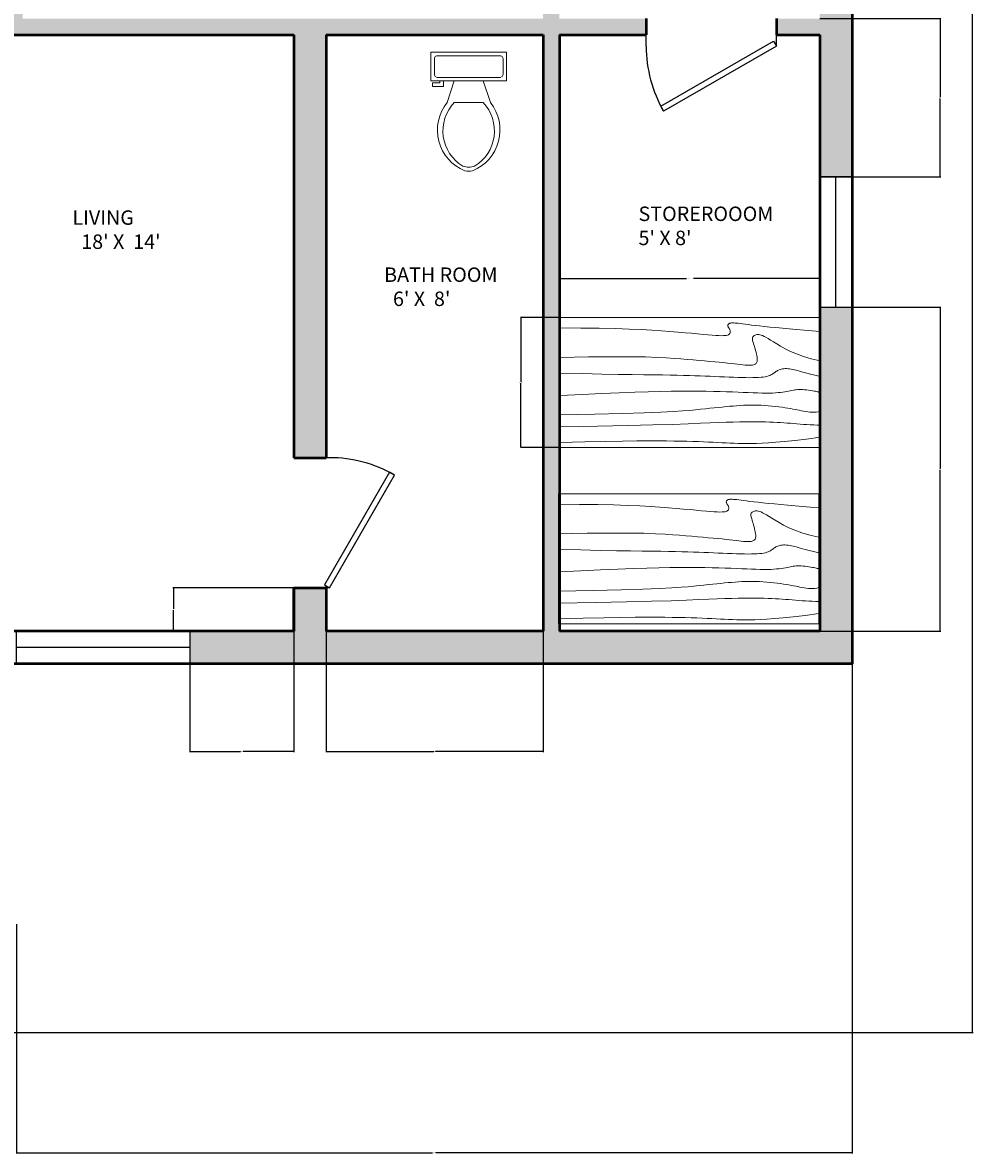
# Model space of a CAD drawing. Units: inches. Extents: x 4 to 671, y -79 to 570.
# Tile 5 of 7: x 408 to 671, y -79 to 234. Entities that reach past the tile are written whole.
import ezdxf

# ---------------------------------------------------------------- set-up
doc = ezdxf.new("R2010")
doc.units = ezdxf.units.IN
doc.header["$MEASUREMENT"] = 0
for name, color, linetype, lineweight in [('A-ANNO-DIMS', 2, 'Continuous', 18), ('A-AREA-IDEN', 7, 'Continuous', 18), ('A-WALL', 7, 'Continuous', 50), ('A-WALL-PATT', 251, 'Continuous', 13), ('bathroom', 90, 'Continuous', 18), ('doors', 40, 'Continuous', 25), ('furniture', 220, 'Continuous', 18), ('window', 30, 'Continuous', 25)]:
    doc.layers.add(name, color=color, linetype=linetype, lineweight=lineweight)
doc.styles.get("Standard").update_dxf_attribs({"font": 'arial.ttf'})
doc.dimstyles.get("Standard").update_dxf_attribs({"dimtxt": 0.18, "dimasz": 0.18, "dimexe": 0.18, "dimexo": 0.0625, "dimgap": 0.09, "dimtad": 0, "dimtih": 1, "dimtoh": 1, "dimdec": 4, "dimzin": 0, "dimdsep": 46, "dimtxsty": 'Standard', "dimcen": 0.09, "dimadec": 0, "dimazin": 0, "dimtfac": 1, "dimtdec": 4, "dimtofl": 0, "dimtmove": 0, "dimatfit": 3, "dimfxl": 1, "dimtolj": 1, "dimtzin": 0, "dimarcsym": 0})

# ---------------------------------------------------------------- blocks, each defined once
blk = doc.blocks.new('*U9')
for p, q in [((0, 0), (0, -6)), ((40, 0), (40, -6))]:
    blk.add_line(p, q)
blk.add_lwpolyline([(0, 0), (34.64, 20), (35.52, 18.48), (0.87, -1.52)], close=True)
blk.add_arc((0, 0), 40, 0, 30)
blk = doc.blocks.new('*U12')
for p, q in [((0, 0), (0, -6)), ((-40, 0), (-40, -6))]:
    blk.add_line(p, q)
blk.add_lwpolyline([(0, 0), (-34.64, 20), (-35.52, 18.48), (-0.88, -1.52)], close=True)
blk.add_arc((0, 0), 40, 150, 180)
blk = doc.blocks.new('Toilet - top')
for p, q in [((9.5, -6), (9.5, -2)), ((-10, -8.5), (-8, -8.5)), ((-10, -9.5), (-10, -8.5)), ((-8, -8.5), (-8, -8)), ((-7, -8), (-7, -9.5)), ((-4, -8), (-6, -14)), ((4, -8), (6, -14)), ((-7, -9.5), (-10, -9.5)), ((4, -14), (-4, -14))]:
    blk.add_line(p, q)
blk.add_lwpolyline([(10.5, -8), (10.5, 0), (-10.5, 0), (-10.5, -8)], close=True)
for points in [[(-9.5, -2), (-9.5, -6)], [(8.5, -1), (-8.5, -1)], [(-8.5, -7), (8.5, -7)]]:
    blk.add_lwpolyline(points)
for centre, radius, start, end in [((-8.62, -1.88), 0.884, 81.8699, 188.1301), ((8.62, -1.88), 0.884, 351.8699, 98.1301), ((-8.62, -6.12), 0.884, 171.8699, 278.1301), ((8.62, -6.12), 0.884, 261.8699, 8.1301), ((3.52, -21.58), 12.17, 141.4691, 247.9714), ((4.2, -21.82), 11.33, 136.3677, 238.9468), ((-3.52, -21.58), 12.17, 292.0284, 38.5307), ((-4.2, -21.82), 11.33, 301.053, 43.6321), ((0, -27.88), 4, 245.7318, 294.2682), ((0, -29), 4, 254.8605, 285.1395)]:
    blk.add_arc(centre, radius, start, end)
blk = doc.blocks.new('Table - Rectangular Woodgrain 60 x 30 in.')
for p, q in [((0, 0), (0, -30)), ((60, 0), (0, 0)), ((60, -30), (60, 0)), ((0, -30), (60, -30))]:
    blk.add_line(p, q)
for points in [[(0, -2.4), (4.8155, -2.418), (9.0302, -2.4688), (12.709, -2.5477), (15.9167, -2.65), (18.7181, -2.7711), (21.1781, -2.9063), (23.3616, -3.0508), (25.3333, -3.2), (27.1477, -3.3495), (28.8172, -3.4958), (30.3437, -3.636), (31.7291, -3.7667), (32.9756, -3.8849), (34.0849, -3.9875), (35.059, -4.0714), (35.9, -4.1334), (36.6114, -4.1711), (37.2041, -4.1854), (37.6906, -4.1779), (38.0833, -4.15), (38.3948, -4.1034), (38.6375, -4.0396), (38.8239, -3.9602), (38.9666, -3.8667), (39.0764, -3.7608), (39.1573, -3.6448), (39.2116, -3.521), (39.2416, -3.3917), (39.2498, -3.2593), (39.2385, -3.1261), (39.21, -2.9944), (39.1666, -2.8667), (39.111, -2.7447), (39.0468, -2.6281), (38.978, -2.5163), (38.9083, -2.4083), (38.8418, -2.3035), (38.7823, -2.201), (38.7337, -2.1001), (38.7, -2), (38.6844, -1.9003), (38.6875, -1.8021), (38.7094, -1.707), (38.75, -1.6167), (38.8094, -1.5326), (38.8875, -1.4563), (38.9844, -1.3893), (39.1, -1.3333), (39.2351, -1.2896), (39.3937, -1.2583), (39.5804, -1.2396), (39.8, -1.2333), (40.057, -1.2396), (40.3562, -1.2583), (40.7023, -1.2896), (41.1, -1.3333), (41.5547, -1.3895), (42.0755, -1.4573), (42.6721, -1.5361), (43.3542, -1.625), (44.1316, -1.7233), (45.014, -1.8302), (46.0114, -1.9449), (47.1333, -2.0667), (48.3862, -2.1947), (49.7625, -2.3281), (51.2513, -2.4663), (52.8416, -2.6083), (54.5226, -2.7535), (56.2833, -2.9011), (58.1127, -3.0501), (60, -3.2)], [(0, -9.2), (6.5759, -9.0858), (11.9385, -9.0365), (16.2527, -9.0418), (19.6833, -9.0917), (22.3952, -9.1759), (24.5531, -9.2844), (26.322, -9.4069), (27.8666, -9.5333), (29.3241, -9.6553), (30.7203, -9.7719), (32.0532, -9.8837), (33.3208, -9.9917), (34.5213, -10.0965), (35.6526, -10.199), (36.7128, -10.2999), (37.7, -10.4), (38.6129, -10.4996), (39.4531, -10.5969), (40.223, -10.6895), (40.925, -10.775), (41.5613, -10.8512), (42.1344, -10.9156), (42.6465, -10.966), (43.1, -11), (43.4976, -11.0158), (43.8437, -11.0136), (44.143, -10.9942), (44.4, -10.9583), (44.6195, -10.9069), (44.8062, -10.8406), (44.9648, -10.7603), (45.1, -10.6667), (45.2155, -10.5598), (45.3114, -10.4365), (45.3871, -10.2929), (45.4416, -10.125), (45.4743, -9.929), (45.4844, -9.7011), (45.4709, -9.4371), (45.4333, -9.1333), (45.3716, -8.7883), (45.2896, -8.4104), (45.1919, -8.0107), (45.0833, -7.6), (44.9685, -7.1893), (44.8521, -6.7896), (44.7388, -6.4117), (44.6333, -6.0667), (44.54, -5.7628), (44.4614, -5.4979), (44.4001, -5.2675), (44.3583, -5.0667), (44.3384, -4.8909), (44.3427, -4.7354), (44.3736, -4.5956), (44.4333, -4.4667), (44.5236, -4.3453), (44.6427, -4.2333), (44.7884, -4.1339), (44.9583, -4.05), (45.1501, -3.9849), (45.3614, -3.9417), (45.59, -3.9234), (45.8333, -3.9333), (46.0915, -3.9749), (46.3734, -4.0531), (46.6906, -4.1736), (47.0542, -4.3417), (47.4756, -4.5629), (47.9661, -4.8427), (48.5372, -5.1866), (49.2, -5.6), (49.9676, -6.0844), (50.8594, -6.625), (51.8965, -7.2031), (53.1, -7.8), (54.491, -8.3969), (56.0906, -8.975), (57.9199, -9.5156), (60, -10)], [(0, -12.8), (5.1847, -12.9322), (9.6213, -13.0323), (13.3963, -13.1059), (16.5958, -13.1583), (19.3063, -13.1952), (21.614, -13.2219), (23.6054, -13.2439), (25.3666, -13.2667), (26.9728, -13.2947), (28.4531, -13.3281), (29.8256, -13.3663), (31.1083, -13.4083), (32.3191, -13.4535), (33.476, -13.501), (34.597, -13.5501), (35.7, -13.6), (36.7984, -13.6497), (37.8875, -13.6979), (38.9578, -13.743), (40, -13.7833), (41.0047, -13.8174), (41.9625, -13.8438), (42.864, -13.8607), (43.7, -13.8667), (44.4631, -13.8604), (45.1552, -13.8417), (45.7801, -13.8104), (46.3416, -13.7667), (46.8439, -13.7104), (47.2906, -13.6417), (47.6858, -13.5604), (48.0333, -13.4667), (48.3375, -13.3608), (48.6042, -13.2448), (48.8396, -13.121), (49.05, -12.9917), (49.2417, -12.8593), (49.4208, -12.7261), (49.5937, -12.5944), (49.7667, -12.4667), (49.9452, -12.3451), (50.1323, -12.2313), (50.3303, -12.1268), (50.5416, -12.0333), (50.7686, -11.9524), (51.0135, -11.8854), (51.2788, -11.8341), (51.5666, -11.8), (51.8785, -11.7843), (52.2116, -11.7865), (52.562, -11.8059), (52.926, -11.8417), (53.2998, -11.8931), (53.6795, -11.9594), (54.0614, -12.0397), (54.4416, -12.1333), (54.8223, -12.2401), (55.2293, -12.3625), (55.6942, -12.5037), (56.2489, -12.6667), (56.9251, -12.8547), (57.7545, -13.0708), (58.7689, -13.3182), (60, -13.6)], [(0, -18), (5.124, -17.7273), (9.6609, -17.5057), (13.6705, -17.3303), (17.2125, -17.1958), (20.3467, -17.0973), (23.1328, -17.0297), (25.6307, -16.9878), (27.9, -16.9667), (29.9928, -16.9617), (31.9302, -16.9703), (33.7254, -16.9907), (35.3917, -17.0208), (36.9423, -17.0588), (38.3906, -17.1026), (39.7499, -17.1503), (41.0333, -17.2), (42.2519, -17.2496), (43.4073, -17.2969), (44.4986, -17.3395), (45.525, -17.375), (46.4858, -17.4012), (47.3802, -17.4156), (48.2074, -17.416), (48.9667, -17.4), (49.6583, -17.3662), (50.2872, -17.3167), (50.8595, -17.2547), (51.3812, -17.1833), (51.8584, -17.1057), (52.2971, -17.025), (52.7034, -16.9443), (53.0833, -16.8667), (53.443, -16.7951), (53.789, -16.7313), (54.128, -16.6768), (54.4666, -16.6334), (54.8115, -16.6024), (55.1693, -16.5854), (55.5465, -16.5841), (55.95, -16.6), (56.3828, -16.6337), (56.8346, -16.6823), (57.2915, -16.7418), (57.7396, -16.8084), (58.165, -16.878), (58.5539, -16.9469), (58.8924, -17.0111), (59.1666, -17.0667), (59.3679, -17.1107), (59.5078, -17.1438), (59.6032, -17.1675), (59.6708, -17.1833), (59.7275, -17.193), (59.7901, -17.1979), (59.8753, -17.1998), (60, -17.2)], [(0, -22.4), (8.0098, -22.2501), (14.4094, -22.1011), (19.4168, -21.9535), (23.25, -21.8083), (26.1269, -21.6663), (28.2656, -21.5281), (29.884, -21.3947), (31.2, -21.2667), (32.3967, -21.1448), (33.5172, -21.0292), (34.5697, -20.9198), (35.5625, -20.8167), (36.5037, -20.7198), (37.4015, -20.6292), (38.2642, -20.5448), (39.1, -20.4667), (39.9164, -20.3951), (40.7187, -20.3313), (41.5117, -20.2768), (42.3, -20.2333), (43.0883, -20.2024), (43.8812, -20.1854), (44.6836, -20.1841), (45.5, -20.2), (46.3328, -20.234), (47.1747, -20.2844), (48.0163, -20.3488), (48.8479, -20.425), (49.66, -20.5106), (50.4429, -20.6031), (51.1872, -20.7004), (51.8833, -20.8), (52.5246, -20.8999), (53.1166, -20.9995), (53.6681, -21.0983), (54.1875, -21.1958), (54.6834, -21.2919), (55.1646, -21.3859), (55.6394, -21.4777), (56.1167, -21.5667), (56.6028, -21.6515), (57.0961, -21.7266), (57.5929, -21.7852), (58.0896, -21.8208), (58.5823, -21.8268), (59.0674, -21.7964), (59.5412, -21.723), (60, -21.6)], [(0, -25.2), (8.6355, -25.0504), (15.7026, -24.9031), (21.4049, -24.7606), (25.9458, -24.625), (29.529, -24.4988), (32.3578, -24.3844), (34.6359, -24.284), (36.5667, -24.2), (38.3213, -24.1341), (39.9417, -24.0854), (41.437, -24.0523), (42.8167, -24.0333), (44.0901, -24.0268), (45.2667, -24.0313), (46.3557, -24.0451), (47.3667, -24.0667), (48.309, -24.0947), (49.1928, -24.1287), (50.0284, -24.168), (50.826, -24.2125), (51.5959, -24.2617), (52.3483, -24.3151), (53.0935, -24.3725), (53.8417, -24.4334), (54.6009, -24.497), (55.3699, -24.561), (56.1454, -24.6226), (56.9239, -24.6792), (57.7021, -24.7279), (58.4764, -24.7662), (59.2435, -24.7911), (60, -24.8)], [(0, -28.8), (5.6867, -28.6681), (10.45, -28.5698), (14.407, -28.5012), (17.675, -28.4584), (20.3711, -28.4374), (22.6125, -28.4344), (24.5164, -28.4455), (26.2, -28.4667), (27.762, -28.4947), (29.2276, -28.5281), (30.6033, -28.5663), (31.8958, -28.6084), (33.1118, -28.6535), (34.2578, -28.7011), (35.3405, -28.7501), (36.3666, -28.8), (37.3443, -28.8497), (38.288, -28.8974), (39.2137, -28.9412), (40.1375, -28.9792), (41.0753, -29.0093), (42.0432, -29.0297), (43.0572, -29.0384), (44.1333, -29.0333), (45.2936, -29.0114), (46.5843, -28.9641), (48.0579, -28.8816), (49.7666, -28.7542), (51.7629, -28.5721), (54.0989, -28.3255), (56.8272, -28.0048), (60, -27.6)]]:
    blk.add_lwpolyline(points)
blk = doc.blocks.new('WIN-36-EAST')
for p, q in [((9, 36), (0, 36)), ((0, 36), (0, 0)), ((4.5, 0), (4.5, 36)), ((9, 0), (9, 36)), ((0, 0), (9, 0)), ((0, 0), (4.5, 0))]:
    blk.add_line(p, q)
blk = doc.blocks.new('WIN-48')
for p, q in [((0, 9), (0, 0)), ((48, 9), (0, 9)), ((0, 9), (0, 4.5)), ((48, 0), (48, 9)), ((0, 4.5), (48, 4.5)), ((0, 0), (48, 0))]:
    blk.add_line(p, q)
blk = doc.blocks.new('*D31')
at = {"layer": 'A-ANNO-DIMS', "color": 0, "lineweight": -2, "transparency": 16777216}
for p, q in [((556.6, 152.19), (556.6, 163.11)), ((556.78, 162.93), (591.63, 162.93)), ((628.42, 162.93), (593.56, 162.93)), ((628.6, 152.19), (628.6, 163.11))]:
    blk.add_line(p, q, dxfattribs=at)
at = {"layer": 'A-ANNO-DIMS', "color": 0, "transparency": 16777216}
for points in [[(556.78, 162.96), (556.78, 162.9), (556.6, 162.93)], [(628.42, 162.96), (628.42, 162.9), (628.6, 162.93)]]:
    blk.add_solid(points, dxfattribs=at)
at = {"layer": 'Defpoints', "color": 0, "transparency": 16777216}
for p in [(628.6, 162.93), (556.6, 152.13), (628.6, 152.13)]:
    blk.add_point(p, dxfattribs=at)
at = {"layer": 'A-ANNO-DIMS', "color": 0, "transparency": 16777216, "insert": (592.6, 162.93), "char_height": 0.18, "attachment_point": 5}
blk.add_mtext('\\A1;TABLE 72 TYP.', dxfattribs=at)
blk = doc.blocks.new('*D32')
at = {"layer": 'A-ANNO-DIMS', "color": 0, "lineweight": -2, "transparency": 16777216}
for p, q in [((556.53, 152.13), (545.62, 152.13)), ((545.8, 151.95), (545.8, 134.31)), ((545.8, 116.31), (545.8, 133.95)), ((556.53, 116.13), (545.62, 116.13))]:
    blk.add_line(p, q, dxfattribs=at)
at = {"layer": 'A-ANNO-DIMS', "color": 0, "transparency": 16777216}
for points in [[(545.77, 151.95), (545.83, 151.95), (545.8, 152.13)], [(545.77, 116.31), (545.83, 116.31), (545.8, 116.13)]]:
    blk.add_solid(points, dxfattribs=at)
at = {"layer": 'Defpoints', "color": 0, "transparency": 16777216}
for p in [(545.8, 152.13), (556.6, 152.13), (556.6, 116.13)]:
    blk.add_point(p, dxfattribs=at)
at = {"layer": 'A-ANNO-DIMS', "color": 0, "transparency": 16777216, "insert": (545.8, 134.13), "char_height": 0.18, "attachment_point": 5}
blk.add_mtext('\\A1;36 TYP.', dxfattribs=at)
blk = doc.blocks.new('*D50')
at = {"layer": 'A-ANNO-DIMS', "color": 0, "lineweight": -2, "transparency": 16777216}
for p, q in [((637.5, 536.35), (670.92, 536.35)), ((670.74, 536.17), (670.74, 245.53)), ((670.74, -45.47), (670.74, 245.17)), ((389.27, -45.65), (670.92, -45.65))]:
    blk.add_line(p, q, dxfattribs=at)
at = {"layer": 'A-ANNO-DIMS', "color": 0, "transparency": 16777216}
for points in [[(670.71, 536.17), (670.77, 536.17), (670.74, 536.35)], [(670.71, -45.47), (670.77, -45.47), (670.74, -45.65)]]:
    blk.add_solid(points, dxfattribs=at)
at = {"layer": 'Defpoints', "color": 0, "transparency": 16777216}
for p in [(637.44, 536.35), (389.21, -45.65), (670.74, -45.65)]:
    blk.add_point(p, dxfattribs=at)
at = {"layer": 'A-ANNO-DIMS', "color": 0, "transparency": 16777216, "insert": (670.74, 245.35), "char_height": 0.18, "attachment_point": 5}
blk.add_mtext('\\A1;582', dxfattribs=at)
blk = doc.blocks.new('*D58')
at = {"layer": 'A-ANNO-DIMS', "color": 0, "lineweight": -2, "transparency": 16777216}
for p, q in [((637.44, 56.29), (637.44, -79.13)), ((406.21, -15.71), (406.21, -79.13)), ((406.39, -78.95), (521.36, -78.95)), ((637.26, -78.95), (522.29, -78.95))]:
    blk.add_line(p, q, dxfattribs=at)
at = {"layer": 'A-ANNO-DIMS', "color": 0, "transparency": 16777216}
for points in [[(406.39, -78.92), (406.39, -78.98), (406.21, -78.95)], [(637.26, -78.92), (637.26, -78.98), (637.44, -78.95)]]:
    blk.add_solid(points, dxfattribs=at)
at = {"layer": 'Defpoints', "color": 0, "transparency": 16777216}
for p in [(637.44, 56.35), (406.21, -15.65), (637.44, -78.95)]:
    blk.add_point(p, dxfattribs=at)
at = {"layer": 'A-ANNO-DIMS', "color": 0, "transparency": 16777216, "insert": (521.82, -78.95), "char_height": 0.18, "attachment_point": 5}
blk.add_mtext('\\A1;231.23', dxfattribs=at)
blk = doc.blocks.new('*D64')
at = {"layer": 'A-ANNO-DIMS', "color": 0, "lineweight": -2, "transparency": 16777216}
for p, q in [((491.94, 65.29), (491.94, 31.87)), ((551.94, 65.29), (551.94, 31.87)), ((492.12, 32.05), (521.72, 32.05)), ((551.76, 32.05), (522.16, 32.05))]:
    blk.add_line(p, q, dxfattribs=at)
at = {"layer": 'A-ANNO-DIMS', "color": 0, "transparency": 16777216}
for points in [[(492.12, 32.08), (492.12, 32.02), (491.94, 32.05)], [(551.76, 32.08), (551.76, 32.02), (551.94, 32.05)]]:
    blk.add_solid(points, dxfattribs=at)
at = {"layer": 'Defpoints', "color": 0, "transparency": 16777216}
for p in [(491.94, 65.35), (551.94, 65.35), (491.94, 32.05)]:
    blk.add_point(p, dxfattribs=at)
at = {"layer": 'A-ANNO-DIMS', "color": 0, "transparency": 16777216, "insert": (521.94, 32.05), "char_height": 0.18, "attachment_point": 5}
blk.add_mtext('\\A1;60', dxfattribs=at)
blk = doc.blocks.new('*D77')
at = {"layer": 'A-ANNO-DIMS', "color": 0, "lineweight": -2, "transparency": 16777216}
for p, q in [((628.5, 234.85), (661.92, 234.85)), ((661.74, 234.67), (661.74, 213.13)), ((661.74, 191.22), (661.74, 212.76)), ((628.5, 191.04), (661.92, 191.04))]:
    blk.add_line(p, q, dxfattribs=at)
at = {"layer": 'A-ANNO-DIMS', "color": 0, "transparency": 16777216}
for points in [[(661.71, 234.67), (661.77, 234.67), (661.74, 234.85)], [(661.71, 191.22), (661.77, 191.22), (661.74, 191.04)]]:
    blk.add_solid(points, dxfattribs=at)
at = {"layer": 'Defpoints', "color": 0, "transparency": 16777216}
for p in [(628.44, 234.85), (628.44, 191.04), (661.74, 191.04)]:
    blk.add_point(p, dxfattribs=at)
at = {"layer": 'A-ANNO-DIMS', "color": 0, "transparency": 16777216, "insert": (661.74, 212.95), "char_height": 0.18, "attachment_point": 5}
blk.add_mtext('\\A1;43.81', dxfattribs=at)
blk = doc.blocks.new('*D78')
at = {"layer": 'A-ANNO-DIMS', "color": 0, "lineweight": -2, "transparency": 16777216}
for p, q in [((628.5, 155.04), (661.92, 155.04)), ((661.74, 154.86), (661.74, 110.38)), ((661.74, 65.53), (661.74, 110.01)), ((628.5, 65.35), (661.92, 65.35))]:
    blk.add_line(p, q, dxfattribs=at)
at = {"layer": 'A-ANNO-DIMS', "color": 0, "transparency": 16777216}
for points in [[(661.71, 154.86), (661.77, 154.86), (661.74, 155.04)], [(661.71, 65.53), (661.77, 65.53), (661.74, 65.35)]]:
    blk.add_solid(points, dxfattribs=at)
at = {"layer": 'Defpoints', "color": 0, "transparency": 16777216}
for p in [(628.44, 155.04), (628.44, 65.35), (661.74, 65.35)]:
    blk.add_point(p, dxfattribs=at)
at = {"layer": 'A-ANNO-DIMS', "color": 0, "transparency": 16777216, "insert": (661.74, 110.2), "char_height": 0.18, "attachment_point": 5}
blk.add_mtext('\\A1;89.69', dxfattribs=at)
blk = doc.blocks.new('*D88')
at = {"layer": 'A-ANNO-DIMS', "color": 0, "lineweight": -2, "transparency": 16777216}
for p, q in [((454.21, 65.29), (454.21, 31.87)), ((482.94, 65.29), (482.94, 31.87)), ((454.39, 32.05), (468.18, 32.05)), ((482.76, 32.05), (468.97, 32.05))]:
    blk.add_line(p, q, dxfattribs=at)
at = {"layer": 'A-ANNO-DIMS', "color": 0, "transparency": 16777216}
for points in [[(454.39, 32.08), (454.39, 32.02), (454.21, 32.05)], [(482.76, 32.08), (482.76, 32.02), (482.94, 32.05)]]:
    blk.add_solid(points, dxfattribs=at)
at = {"layer": 'Defpoints', "color": 0, "transparency": 16777216}
for p in [(454.21, 65.35), (482.94, 65.35), (454.21, 32.05)]:
    blk.add_point(p, dxfattribs=at)
at = {"layer": 'A-ANNO-DIMS', "color": 0, "transparency": 16777216, "insert": (468.57, 32.05), "char_height": 0.18, "attachment_point": 5}
blk.add_mtext('\\A1;28.73', dxfattribs=at)
blk = doc.blocks.new('*D96')
at = {"layer": 'A-ANNO-DIMS', "color": 0, "lineweight": -2, "transparency": 16777216}
for p, q in [((482.88, 77.35), (449.46, 77.35)), ((449.64, 77.17), (449.64, 71.53)), ((449.64, 65.53), (449.64, 71.17)), ((482.88, 65.35), (449.46, 65.35))]:
    blk.add_line(p, q, dxfattribs=at)
at = {"layer": 'A-ANNO-DIMS', "color": 0, "transparency": 16777216}
for points in [[(449.61, 77.17), (449.67, 77.17), (449.64, 77.35)], [(449.61, 65.53), (449.67, 65.53), (449.64, 65.35)]]:
    blk.add_solid(points, dxfattribs=at)
at = {"layer": 'Defpoints', "color": 0, "transparency": 16777216}
for p in [(449.64, 77.35), (482.94, 77.35), (482.94, 65.35)]:
    blk.add_point(p, dxfattribs=at)
at = {"layer": 'A-ANNO-DIMS', "color": 0, "transparency": 16777216, "insert": (449.64, 71.35), "char_height": 0.18, "attachment_point": 5}
blk.add_mtext('\\A1;12', dxfattribs=at)

msp = doc.modelspace()

# ---------------------------------------------------------------- hatches: boundary and pattern name
at = {"layer": 'A-WALL-PATT'}
h = msp.add_hatch(color=256, dxfattribs=at)
h.dxf.hatch_style = 1
h.paths.add_polyline_path([(637.4392, 306.8513), (628.4392, 306.8513), (628.4392, 234.8513), (616.4392, 234.8513), (616.4392, 230.3513), (628.4392, 230.3513), (628.4392, 191.0418), (637.4392, 191.0418)])
h.paths.add_polyline_path([(491.9392, 230.3513), (551.9392, 230.3513), (551.9392, 65.3513), (491.9392, 65.3513), (491.9392, 77.3513), (482.9392, 77.3513), (482.9392, 65.3513), (454.2077, 65.3513), (454.2077, 60.8513), (454.2077, 56.3513), (637.4392, 56.3513), (637.4392, 155.0418), (628.4392, 155.0418), (628.4392, 65.3513), (556.4392, 65.3513), (556.4392, 230.3513), (580.4392, 230.3513), (580.4392, 234.8513), (556.4392, 234.8513), (556.4392, 254.3513), (551.9002, 254.3513), (551.9002, 234.8513), (407.9392, 234.8513), (407.9392, 246.8513), (403.4392, 246.8513), (403.4392, 230.3513), (482.9392, 230.3513), (482.9392, 113.3513), (491.9392, 113.3513)])

# ---------------------------------------------------------------- linework, layer by layer
at = {"layer": 'A-WALL'}
for p, q in [((580.4392, 234.8513), (580.4392, 230.3513)), ((616.4392, 234.8513), (616.4392, 230.3513)), ((403.4392, 230.3513), (482.9392, 230.3513)), ((482.9392, 230.3513), (482.9392, 113.3513)), ((491.9392, 230.3513), (551.9392, 230.3513)), ((491.9392, 230.3513), (491.9392, 113.3513)), ((551.9392, 230.3513), (551.9392, 65.3513)), ((556.4392, 230.3513), (580.4392, 230.3513)), ((556.4392, 230.3513), (556.4392, 65.3513)), ((616.4392, 230.3513), (628.4392, 230.3513)), ((628.4392, 230.3513), (628.4392, 65.3513)), ((482.9392, 113.3513), (491.9392, 113.3513)), ((482.9392, 77.3513), (482.9392, 65.3513)), ((482.9392, 65.3513), (482.9392, 77.3513)), ((482.9392, 77.3513), (491.9392, 77.3513)), ((491.9392, 77.3513), (491.9392, 65.3513)), ((482.9392, 65.3513), (362.9392, 65.3513)), ((551.9392, 65.3513), (491.9392, 65.3513)), ((628.4392, 65.3513), (556.4392, 65.3513))]:
    msp.add_line(p, q, dxfattribs=at)
msp.add_lwpolyline([(313.4392, 56.3513), (37.4392, 56.3513), (37.4392, 536.3513), (637.4392, 536.3513), (637.4392, 56.3513), (362.9392, 56.3513)], dxfattribs=at)

# ---------------------------------------------------------------- block references
at = {"layer": 'bathroom'}
msp.add_blockref('Toilet - top', (531.3368, 225.5803), dxfattribs=at)
at = {"layer": 'doors', "xscale": 0.9, "yscale": 0.9, "zscale": 0.9}
for name, p, rotation in [('*U9', (616.4392, 227.2013), 180), ('*U12', (492.8392, 77.3513), 269.9999999999769)]:
    msp.add_blockref(name, p, dxfattribs=dict(at, rotation=rotation))
at = {"layer": 'furniture', "xscale": 1.199999999999999, "yscale": 1.199999999999999, "zscale": 1.199999999999999}
for p in [(556.5975, 152.1275), (556.1768, 103.34)]:
    msp.add_blockref('Table - Rectangular Woodgrain 60 x 30 in.', p, dxfattribs=at)
at = {"layer": 'window'}
msp.add_blockref('WIN-36-EAST', (628.439, 155.0415), dxfattribs=at)
at = {"layer": 'window', "extrusion": (0, 0, -1), "zscale": -1}
msp.add_blockref('WIN-48', (-454.2074, 56.351), dxfattribs=at)

# ---------------------------------------------------------------- texts
at = {"layer": 'A-AREA-IDEN', "char_height": 4, "attachment_point": 1}
for s, insert in [("LIVING\\P  18' X  14'", (421.7106, 181.7794)), (" STOREROOOM\\P 5' X 8'", (577.0885, 182.8315)), ("BATH ROOM\\P  6' X  8'", (507.9408, 165.9846))]:
    msp.add_mtext_dynamic_manual_height_columns(s, width=44.806469, gutter_width=1, heights=[0], dxfattribs=dict(at, insert=insert))

# ---------------------------------------------------------------- dimensions: what is measured, and where the dimension line sits
at = {"layer": 'A-ANNO-DIMS'}
for base, p1, p2, angle, override, picture, middle in [((670.7392, -45.6487), (637.4392, 536.3513), (389.2077, -45.6487), 90, {"dimdec": 0, "dimlfac": 1, "dimrnd": 0, "dimzin": 0, "dimdsep": 46, "dimlunit": 2}, '*D50', (670.7392, 245.3513)), ((661.7392, 191.0418), (628.4392, 234.8513), (628.4392, 191.0418), 270, {"dimdec": 2, "dimlfac": 1, "dimrnd": 0, "dimzin": 0, "dimdsep": 46, "dimlunit": 2}, '*D77', (661.7392, 212.9466)), ((661.7392, 65.3513), (628.4392, 155.0418), (628.4392, 65.3513), 270, {"dimdec": 2, "dimlfac": 1, "dimrnd": 0, "dimzin": 0, "dimdsep": 46, "dimlunit": 2}, '*D78', (661.7392, 110.1966)), ((449.6392, 77.3513), (482.9392, 65.3513), (482.9392, 77.3513), 90, {"dimdec": 0, "dimlfac": 1, "dimrnd": 0, "dimzin": 0, "dimdsep": 46, "dimlunit": 2}, '*D96', (449.6392, 71.3513)), ((454.2077, 32.0513), (482.9392, 65.3513), (454.2077, 65.3513), 180, {"dimdec": 2, "dimlfac": 1, "dimrnd": 0, "dimzin": 0, "dimdsep": 46, "dimlunit": 2}, '*D88', (468.5735, 32.0513)), ((491.9392, 32.0513), (551.9392, 65.3513), (491.9392, 65.3513), 180, {"dimdec": 0, "dimlfac": 1, "dimrnd": 0, "dimzin": 0, "dimdsep": 46, "dimlunit": 2}, '*D64', (521.9392, 32.0513))]:
    dim = msp.add_linear_dim(base=base, p1=p1, p2=p2, angle=angle, dimstyle='Standard', override=override, dxfattribs=at)
    dim.commit()
    dim.dimension.update_dxf_attribs({"geometry": picture, "text_midpoint": middle})
dim = msp.add_linear_dim(base=(628.5975, 162.9275), p1=(556.5975, 152.1275), p2=(628.5975, 152.1275), text='TABLE <> TYP.', dimstyle='Standard', override={"dimdec": 0, "dimlfac": 1, "dimrnd": 0, "dimzin": 0, "dimdsep": 46, "dimlunit": 2}, dxfattribs=at)
dim.commit()
dim.dimension.update_dxf_attribs({"geometry": '*D31', "text_midpoint": (592.5975, 162.9275)})
dim = msp.add_linear_dim(base=(545.7975, 152.1275), p1=(556.5975, 116.1275), p2=(556.5975, 152.1275), angle=90, text='<> TYP.', dimstyle='Standard', override={"dimdec": 0, "dimlfac": 1, "dimrnd": 0, "dimzin": 0, "dimdsep": 46, "dimlunit": 2}, dxfattribs=at)
dim.commit()
dim.dimension.update_dxf_attribs({"geometry": '*D32', "text_midpoint": (545.7975, 134.1275)})
dim = msp.add_linear_dim(base=(637.4392, -78.9487), p1=(406.2077, -15.6487), p2=(637.4392, 56.3513), dimstyle='Standard', override={"dimdec": 2, "dimlfac": 1, "dimrnd": 0, "dimzin": 0, "dimdsep": 46, "dimlunit": 2}, dxfattribs=at)
dim.commit()
dim.dimension.update_dxf_attribs({"geometry": '*D58', "text_midpoint": (521.8235, -78.9487)})

doc.saveas('drawing.dxf')
